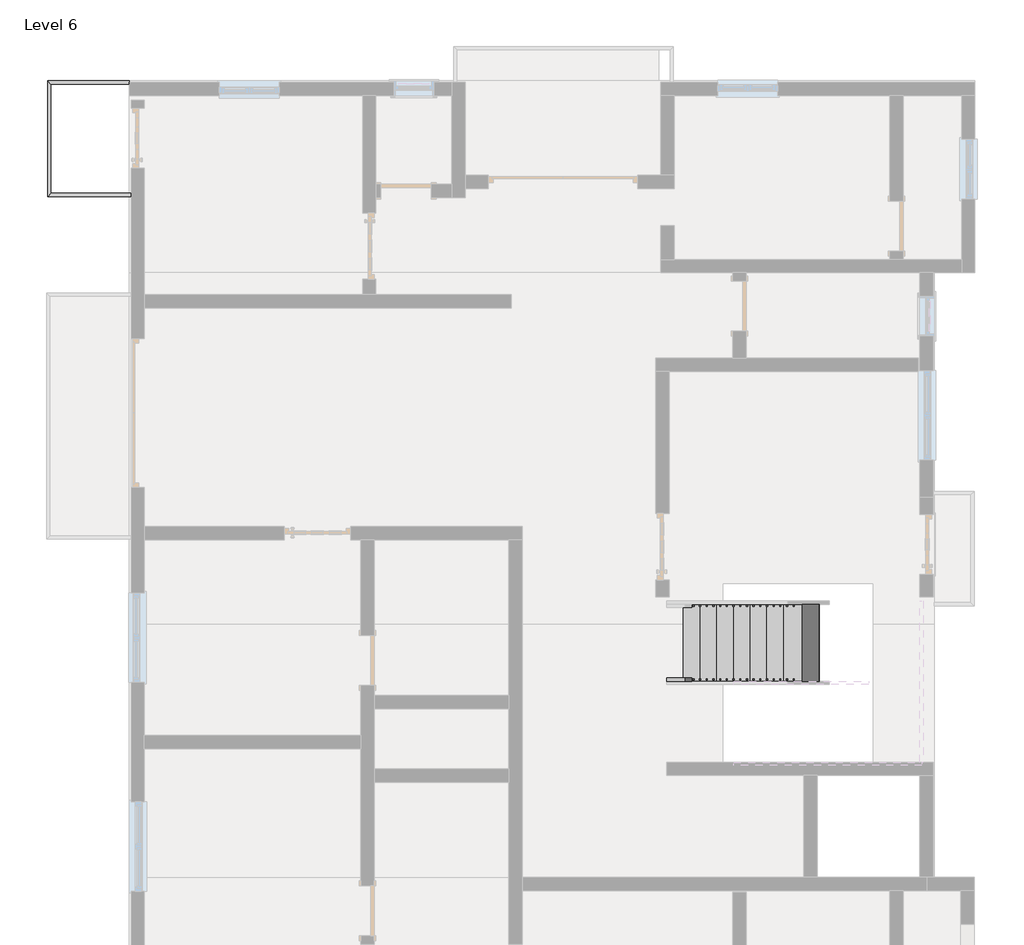
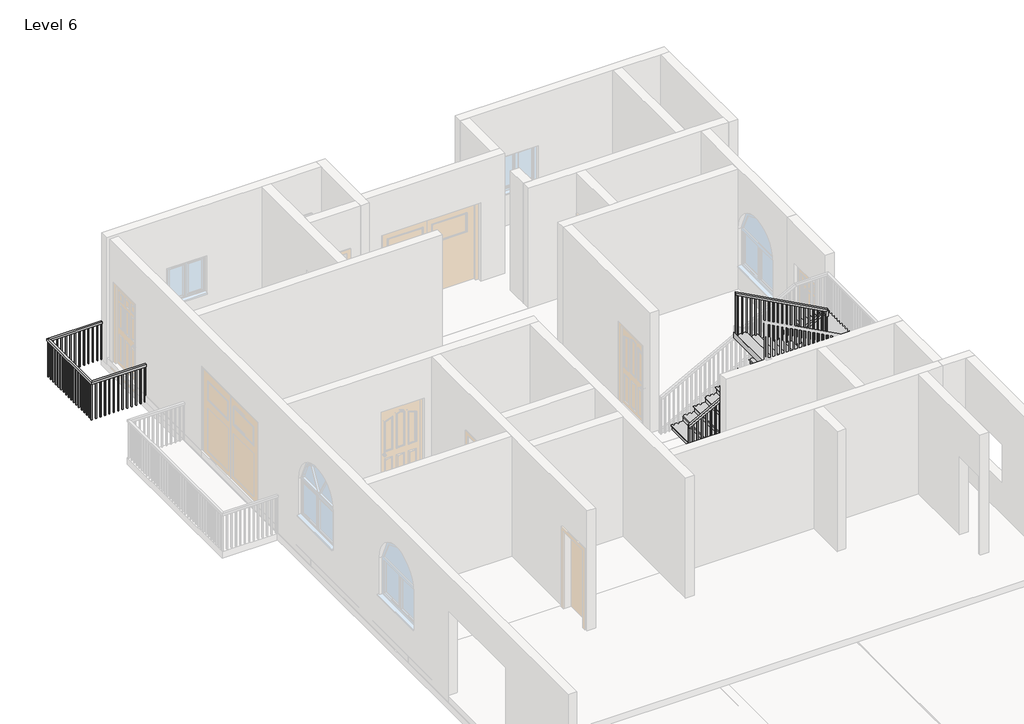
# One storey, part 5 of 7: 2 railings, 1 stair flight.
"""IFC4 building model written with IfcOpenShell, lengths in millimetres."""

from ifc_helpers import new_model, si_unit, frame, origin, place, context, project, spatial, polyline, outline, extrude, faceted_brep, transform, mapped, element, save
from components import stair_flight_0bd31da3

model = new_model("IFC4")

# Units and contexts
model_context = context("Model", 3, world=origin())
ifc_project = project(units=[si_unit("LENGTHUNIT", "METRE", prefix="MILLI")], contexts=[model_context])

# Site, building, storey
site = spatial("IfcSite", under=ifc_project)
building = spatial("IfcBuilding", under=site)
storey = spatial("IfcBuildingStorey", under=building, Name="Level 6", Elevation=15240.0)

# Railings
placement = place(None, origin())
element("IfcRailing", 1, ObjectType="Handrail - Rectangular", at=placement, inside=storey, context=model_context, shape_type="SolidModel", body=[
    faceted_brep([(-6354.2109037, 9376.4527313, 16154.4), (-6354.2109037, 9376.4527313, 16103.6), (-6354.2109037, 9427.2527313, 16103.6), (-6354.2109037, 9427.2527313, 16154.4), (-7548.0109037, 9376.4527313, 16154.4), (-7548.0109037, 9376.4527313, 16103.6), (-7598.8109037, 9427.2527313, 16103.6), (-7598.8109037, 9427.2527313, 16154.4), (-7548.0109037, 7717.9584215, 16154.4), (-7548.0109037, 7717.9584215, 16103.6), (-7598.8109037, 7667.1584215, 16103.6), (-7598.8109037, 7667.1584215, 16154.4), (-6330.8013636, 7717.9584215, 16154.4), (-6330.8013636, 7667.1584215, 16154.4), (-6330.8013636, 7667.1584215, 16103.6), (-6330.8013636, 7717.9584215, 16103.6)], [[[0, 1, 2, 3]], [[1, 0, 4, 5]], [[2, 1, 5, 6]], [[3, 2, 6, 7]], [[0, 3, 7, 4]], [[5, 4, 8, 9]], [[6, 5, 9, 10]], [[7, 6, 10, 11]], [[4, 7, 11, 8]], [[12, 13, 14, 15]], [[9, 8, 12, 15]], [[10, 9, 15, 14]], [[11, 10, 14, 13]], [[8, 11, 13, 12]]]),
    extrude(outline(polyline([(-6363.7359037, 7683.0334215), (-6363.7359037, 7702.0834215), (-6344.6859037, 7702.0834215), (-6344.6859037, 7683.0334215), (-6363.7359037, 7683.0334215)])), frame((0.0, 0.0, 15240.0), z_axis=(0.0, 0.0, 1.0), x_axis=(1.0, 0.0, 0.0)), (0.0, 0.0, 1.0), 863.6),
    extrude(outline(polyline([(-6465.3359037, 7683.0334215), (-6465.3359037, 7702.0834215), (-6446.2859037, 7702.0834215), (-6446.2859037, 7683.0334215), (-6465.3359037, 7683.0334215)])), frame((0.0, 0.0, 15240.0), z_axis=(0.0, 0.0, 1.0), x_axis=(1.0, 0.0, 0.0)), (0.0, 0.0, 1.0), 863.6),
    extrude(outline(polyline([(-6566.9359037, 7683.0334215), (-6566.9359037, 7702.0834215), (-6547.8859037, 7702.0834215), (-6547.8859037, 7683.0334215), (-6566.9359037, 7683.0334215)])), frame((0.0, 0.0, 15240.0), z_axis=(0.0, 0.0, 1.0), x_axis=(1.0, 0.0, 0.0)), (0.0, 0.0, 1.0), 863.6),
    extrude(outline(polyline([(-6668.5359037, 7683.0334215), (-6668.5359037, 7702.0834215), (-6649.4859037, 7702.0834215), (-6649.4859037, 7683.0334215), (-6668.5359037, 7683.0334215)])), frame((0.0, 0.0, 15240.0), z_axis=(0.0, 0.0, 1.0), x_axis=(1.0, 0.0, 0.0)), (0.0, 0.0, 1.0), 863.6),
    extrude(outline(polyline([(-6770.1359037, 7683.0334215), (-6770.1359037, 7702.0834215), (-6751.0859037, 7702.0834215), (-6751.0859037, 7683.0334215), (-6770.1359037, 7683.0334215)])), frame((0.0, 0.0, 15240.0), z_axis=(0.0, 0.0, 1.0), x_axis=(1.0, 0.0, 0.0)), (0.0, 0.0, 1.0), 863.6),
    extrude(outline(polyline([(-6871.7359037, 7683.0334215), (-6871.7359037, 7702.0834215), (-6852.6859037, 7702.0834215), (-6852.6859037, 7683.0334215), (-6871.7359037, 7683.0334215)])), frame((0.0, 0.0, 15240.0), z_axis=(0.0, 0.0, 1.0), x_axis=(1.0, 0.0, 0.0)), (0.0, 0.0, 1.0), 863.6),
    extrude(outline(polyline([(-6973.3359037, 7683.0334215), (-6973.3359037, 7702.0834215), (-6954.2859037, 7702.0834215), (-6954.2859037, 7683.0334215), (-6973.3359037, 7683.0334215)])), frame((0.0, 0.0, 15240.0), z_axis=(0.0, 0.0, 1.0), x_axis=(1.0, 0.0, 0.0)), (0.0, 0.0, 1.0), 863.6),
    extrude(outline(polyline([(-7074.9359037, 7683.0334215), (-7074.9359037, 7702.0834215), (-7055.8859037, 7702.0834215), (-7055.8859037, 7683.0334215), (-7074.9359037, 7683.0334215)])), frame((0.0, 0.0, 15240.0), z_axis=(0.0, 0.0, 1.0), x_axis=(1.0, 0.0, 0.0)), (0.0, 0.0, 1.0), 863.6),
    extrude(outline(polyline([(-7176.5359037, 7683.0334215), (-7176.5359037, 7702.0834215), (-7157.4859037, 7702.0834215), (-7157.4859037, 7683.0334215), (-7176.5359037, 7683.0334215)])), frame((0.0, 0.0, 15240.0), z_axis=(0.0, 0.0, 1.0), x_axis=(1.0, 0.0, 0.0)), (0.0, 0.0, 1.0), 863.6),
    extrude(outline(polyline([(-7278.1359037, 7683.0334215), (-7278.1359037, 7702.0834215), (-7259.0859037, 7702.0834215), (-7259.0859037, 7683.0334215), (-7278.1359037, 7683.0334215)])), frame((0.0, 0.0, 15240.0), z_axis=(0.0, 0.0, 1.0), x_axis=(1.0, 0.0, 0.0)), (0.0, 0.0, 1.0), 863.6),
    extrude(outline(polyline([(-7379.7359037, 7683.0334215), (-7379.7359037, 7702.0834215), (-7360.6859037, 7702.0834215), (-7360.6859037, 7683.0334215), (-7379.7359037, 7683.0334215)])), frame((0.0, 0.0, 15240.0), z_axis=(0.0, 0.0, 1.0), x_axis=(1.0, 0.0, 0.0)), (0.0, 0.0, 1.0), 863.6),
    extrude(outline(polyline([(-7481.3359037, 7683.0334215), (-7481.3359037, 7702.0834215), (-7462.2859037, 7702.0834215), (-7462.2859037, 7683.0334215), (-7481.3359037, 7683.0334215)])), frame((0.0, 0.0, 15240.0), z_axis=(0.0, 0.0, 1.0), x_axis=(1.0, 0.0, 0.0)), (0.0, 0.0, 1.0), 863.6),
    extrude(outline(polyline([(-7582.9359037, 7785.7777313), (-7563.8859037, 7785.7777313), (-7563.8859037, 7766.7277313), (-7582.9359037, 7766.7277313), (-7582.9359037, 7785.7777313)])), frame((0.0, 0.0, 15240.0), z_axis=(0.0, 0.0, 1.0), x_axis=(1.0, 0.0, 0.0)), (0.0, 0.0, 1.0), 863.6),
    extrude(outline(polyline([(-7582.9359037, 7887.3777313), (-7563.8859037, 7887.3777313), (-7563.8859037, 7868.3277313), (-7582.9359037, 7868.3277313), (-7582.9359037, 7887.3777313)])), frame((0.0, 0.0, 15240.0), z_axis=(0.0, 0.0, 1.0), x_axis=(1.0, 0.0, 0.0)), (0.0, 0.0, 1.0), 863.6),
    extrude(outline(polyline([(-7582.9359037, 7988.9777313), (-7563.8859037, 7988.9777313), (-7563.8859037, 7969.9277313), (-7582.9359037, 7969.9277313), (-7582.9359037, 7988.9777313)])), frame((0.0, 0.0, 15240.0), z_axis=(0.0, 0.0, 1.0), x_axis=(1.0, 0.0, 0.0)), (0.0, 0.0, 1.0), 863.6),
    extrude(outline(polyline([(-7582.9359037, 8090.5777313), (-7563.8859037, 8090.5777313), (-7563.8859037, 8071.5277313), (-7582.9359037, 8071.5277313), (-7582.9359037, 8090.5777313)])), frame((0.0, 0.0, 15240.0), z_axis=(0.0, 0.0, 1.0), x_axis=(1.0, 0.0, 0.0)), (0.0, 0.0, 1.0), 863.6),
    extrude(outline(polyline([(-7582.9359037, 8192.1777313), (-7563.8859037, 8192.1777313), (-7563.8859037, 8173.1277313), (-7582.9359037, 8173.1277313), (-7582.9359037, 8192.1777313)])), frame((0.0, 0.0, 15240.0), z_axis=(0.0, 0.0, 1.0), x_axis=(1.0, 0.0, 0.0)), (0.0, 0.0, 1.0), 863.6),
    extrude(outline(polyline([(-7582.9359037, 8293.7777313), (-7563.8859037, 8293.7777313), (-7563.8859037, 8274.7277313), (-7582.9359037, 8274.7277313), (-7582.9359037, 8293.7777313)])), frame((0.0, 0.0, 15240.0), z_axis=(0.0, 0.0, 1.0), x_axis=(1.0, 0.0, 0.0)), (0.0, 0.0, 1.0), 863.6),
    extrude(outline(polyline([(-7582.9359037, 8395.3777313), (-7563.8859037, 8395.3777313), (-7563.8859037, 8376.3277313), (-7582.9359037, 8376.3277313), (-7582.9359037, 8395.3777313)])), frame((0.0, 0.0, 15240.0), z_axis=(0.0, 0.0, 1.0), x_axis=(1.0, 0.0, 0.0)), (0.0, 0.0, 1.0), 863.6),
    extrude(outline(polyline([(-7582.9359037, 8496.9777313), (-7563.8859037, 8496.9777313), (-7563.8859037, 8477.9277313), (-7582.9359037, 8477.9277313), (-7582.9359037, 8496.9777313)])), frame((0.0, 0.0, 15240.0), z_axis=(0.0, 0.0, 1.0), x_axis=(1.0, 0.0, 0.0)), (0.0, 0.0, 1.0), 863.6),
    extrude(outline(polyline([(-7582.9359037, 8598.5777313), (-7563.8859037, 8598.5777313), (-7563.8859037, 8579.5277313), (-7582.9359037, 8579.5277313), (-7582.9359037, 8598.5777313)])), frame((0.0, 0.0, 15240.0), z_axis=(0.0, 0.0, 1.0), x_axis=(1.0, 0.0, 0.0)), (0.0, 0.0, 1.0), 863.6),
    extrude(outline(polyline([(-7582.9359037, 8700.1777313), (-7563.8859037, 8700.1777313), (-7563.8859037, 8681.1277313), (-7582.9359037, 8681.1277313), (-7582.9359037, 8700.1777313)])), frame((0.0, 0.0, 15240.0), z_axis=(0.0, 0.0, 1.0), x_axis=(1.0, 0.0, 0.0)), (0.0, 0.0, 1.0), 863.6),
    extrude(outline(polyline([(-7582.9359037, 8801.7777313), (-7563.8859037, 8801.7777313), (-7563.8859037, 8782.7277313), (-7582.9359037, 8782.7277313), (-7582.9359037, 8801.7777313)])), frame((0.0, 0.0, 15240.0), z_axis=(0.0, 0.0, 1.0), x_axis=(1.0, 0.0, 0.0)), (0.0, 0.0, 1.0), 863.6),
    extrude(outline(polyline([(-7582.9359037, 8903.3777313), (-7563.8859037, 8903.3777313), (-7563.8859037, 8884.3277313), (-7582.9359037, 8884.3277313), (-7582.9359037, 8903.3777313)])), frame((0.0, 0.0, 15240.0), z_axis=(0.0, 0.0, 1.0), x_axis=(1.0, 0.0, 0.0)), (0.0, 0.0, 1.0), 863.6),
    extrude(outline(polyline([(-7582.9359037, 9004.9777313), (-7563.8859037, 9004.9777313), (-7563.8859037, 8985.9277313), (-7582.9359037, 8985.9277313), (-7582.9359037, 9004.9777313)])), frame((0.0, 0.0, 15240.0), z_axis=(0.0, 0.0, 1.0), x_axis=(1.0, 0.0, 0.0)), (0.0, 0.0, 1.0), 863.6),
    extrude(outline(polyline([(-7582.9359037, 9106.5777313), (-7563.8859037, 9106.5777313), (-7563.8859037, 9087.5277313), (-7582.9359037, 9087.5277313), (-7582.9359037, 9106.5777313)])), frame((0.0, 0.0, 15240.0), z_axis=(0.0, 0.0, 1.0), x_axis=(1.0, 0.0, 0.0)), (0.0, 0.0, 1.0), 863.6),
    extrude(outline(polyline([(-7582.9359037, 9208.1777313), (-7563.8859037, 9208.1777313), (-7563.8859037, 9189.1277313), (-7582.9359037, 9189.1277313), (-7582.9359037, 9208.1777313)])), frame((0.0, 0.0, 15240.0), z_axis=(0.0, 0.0, 1.0), x_axis=(1.0, 0.0, 0.0)), (0.0, 0.0, 1.0), 863.6),
    extrude(outline(polyline([(-7582.9359037, 9309.7777313), (-7563.8859037, 9309.7777313), (-7563.8859037, 9290.7277313), (-7582.9359037, 9290.7277313), (-7582.9359037, 9309.7777313)])), frame((0.0, 0.0, 15240.0), z_axis=(0.0, 0.0, 1.0), x_axis=(1.0, 0.0, 0.0)), (0.0, 0.0, 1.0), 863.6),
    extrude(outline(polyline([(-7462.2859037, 9411.3777313), (-7462.2859037, 9392.3277313), (-7481.3359037, 9392.3277313), (-7481.3359037, 9411.3777313), (-7462.2859037, 9411.3777313)])), frame((0.0, 0.0, 15240.0), z_axis=(0.0, 0.0, 1.0), x_axis=(1.0, 0.0, 0.0)), (0.0, 0.0, 1.0), 863.6),
    extrude(outline(polyline([(-7360.6859037, 9411.3777313), (-7360.6859037, 9392.3277313), (-7379.7359037, 9392.3277313), (-7379.7359037, 9411.3777313), (-7360.6859037, 9411.3777313)])), frame((0.0, 0.0, 15240.0), z_axis=(0.0, 0.0, 1.0), x_axis=(1.0, 0.0, 0.0)), (0.0, 0.0, 1.0), 863.6),
    extrude(outline(polyline([(-7259.0859037, 9411.3777313), (-7259.0859037, 9392.3277313), (-7278.1359037, 9392.3277313), (-7278.1359037, 9411.3777313), (-7259.0859037, 9411.3777313)])), frame((0.0, 0.0, 15240.0), z_axis=(0.0, 0.0, 1.0), x_axis=(1.0, 0.0, 0.0)), (0.0, 0.0, 1.0), 863.6),
    extrude(outline(polyline([(-7157.4859037, 9411.3777313), (-7157.4859037, 9392.3277313), (-7176.5359037, 9392.3277313), (-7176.5359037, 9411.3777313), (-7157.4859037, 9411.3777313)])), frame((0.0, 0.0, 15240.0), z_axis=(0.0, 0.0, 1.0), x_axis=(1.0, 0.0, 0.0)), (0.0, 0.0, 1.0), 863.6),
    extrude(outline(polyline([(-7055.8859037, 9411.3777313), (-7055.8859037, 9392.3277313), (-7074.9359037, 9392.3277313), (-7074.9359037, 9411.3777313), (-7055.8859037, 9411.3777313)])), frame((0.0, 0.0, 15240.0), z_axis=(0.0, 0.0, 1.0), x_axis=(1.0, 0.0, 0.0)), (0.0, 0.0, 1.0), 863.6),
    extrude(outline(polyline([(-6954.2859037, 9411.3777313), (-6954.2859037, 9392.3277313), (-6973.3359037, 9392.3277313), (-6973.3359037, 9411.3777313), (-6954.2859037, 9411.3777313)])), frame((0.0, 0.0, 15240.0), z_axis=(0.0, 0.0, 1.0), x_axis=(1.0, 0.0, 0.0)), (0.0, 0.0, 1.0), 863.6),
    extrude(outline(polyline([(-6852.6859037, 9411.3777313), (-6852.6859037, 9392.3277313), (-6871.7359037, 9392.3277313), (-6871.7359037, 9411.3777313), (-6852.6859037, 9411.3777313)])), frame((0.0, 0.0, 15240.0), z_axis=(0.0, 0.0, 1.0), x_axis=(1.0, 0.0, 0.0)), (0.0, 0.0, 1.0), 863.6),
    extrude(outline(polyline([(-6751.0859037, 9411.3777313), (-6751.0859037, 9392.3277313), (-6770.1359037, 9392.3277313), (-6770.1359037, 9411.3777313), (-6751.0859037, 9411.3777313)])), frame((0.0, 0.0, 15240.0), z_axis=(0.0, 0.0, 1.0), x_axis=(1.0, 0.0, 0.0)), (0.0, 0.0, 1.0), 863.6),
    extrude(outline(polyline([(-6649.4859037, 9411.3777313), (-6649.4859037, 9392.3277313), (-6668.5359037, 9392.3277313), (-6668.5359037, 9411.3777313), (-6649.4859037, 9411.3777313)])), frame((0.0, 0.0, 15240.0), z_axis=(0.0, 0.0, 1.0), x_axis=(1.0, 0.0, 0.0)), (0.0, 0.0, 1.0), 863.6),
    extrude(outline(polyline([(-6547.8859037, 9411.3777313), (-6547.8859037, 9392.3277313), (-6566.9359037, 9392.3277313), (-6566.9359037, 9411.3777313), (-6547.8859037, 9411.3777313)])), frame((0.0, 0.0, 15240.0), z_axis=(0.0, 0.0, 1.0), x_axis=(1.0, 0.0, 0.0)), (0.0, 0.0, 1.0), 863.6),
    extrude(outline(polyline([(-6446.2859037, 9411.3777313), (-6446.2859037, 9392.3277313), (-6465.3359037, 9392.3277313), (-6465.3359037, 9411.3777313), (-6446.2859037, 9411.3777313)])), frame((0.0, 0.0, 15240.0), z_axis=(0.0, 0.0, 1.0), x_axis=(1.0, 0.0, 0.0)), (0.0, 0.0, 1.0), 863.6),
    extrude(outline(polyline([(-7582.9359037, 7702.0834215), (-7563.8859037, 7702.0834215), (-7563.8859037, 7683.0334215), (-7582.9359037, 7683.0334215), (-7582.9359037, 7702.0834215)])), frame((0.0, 0.0, 15240.0), z_axis=(0.0, 0.0, 1.0), x_axis=(1.0, 0.0, 0.0)), (0.0, 0.0, 1.0), 863.6),
    extrude(outline(polyline([(-7563.8859037, 9411.3777313), (-7563.8859037, 9392.3277313), (-7582.9359037, 9392.3277313), (-7582.9359037, 9411.3777313), (-7563.8859037, 9411.3777313)])), frame((0.0, 0.0, 15240.0), z_axis=(0.0, 0.0, 1.0), x_axis=(1.0, 0.0, 0.0)), (0.0, 0.0, 1.0), 863.6),
    extrude(outline(polyline([(-6349.8513636, 7683.0334215), (-6349.8513636, 7702.0834215), (-6330.8013636, 7702.0834215), (-6330.8013636, 7683.0334215), (-6349.8513636, 7683.0334215)])), frame((0.0, 0.0, 15240.0), z_axis=(0.0, 0.0, 1.0), x_axis=(1.0, 0.0, 0.0)), (0.0, 0.0, 1.0), 863.6),
    extrude(outline(polyline([(-6354.2109037, 9411.3777313), (-6354.2109037, 9392.3277313), (-6373.2609037, 9392.3277313), (-6373.2609037, 9411.3777313), (-6354.2109037, 9411.3777313)])), frame((0.0, 0.0, 15240.0), z_axis=(0.0, 0.0, 1.0), x_axis=(1.0, 0.0, 0.0)), (0.0, 0.0, 1.0), 863.6),
])
element("IfcRailing", 2, ObjectType="Handrail - Rectangular", at=placement, inside=storey, context=model_context, shape_type="SolidModel", body=[
    faceted_brep([(1811.8890963, 347.1962251, 16292.9454545), (1811.8890963, 347.1962251, 16235.1709673), (1811.8890963, 296.3962251, 16235.1709673), (1811.8890963, 296.3962251, 16292.9454545), (4804.8326586, 347.1962251, 17914.2136078), (4855.6326586, 347.1962251, 17883.9573214), (4855.6326586, 296.3962251, 17883.9573214), (4804.8326586, 296.3962251, 17914.2136078), (4804.8326586, 347.1962251, 17955.4909091), (4855.6326586, 347.1962251, 17904.6909091), (4855.6326586, 296.3962251, 17904.6909091), (4804.8326586, 296.3962251, 17955.4909091), (4931.8326586, 347.1962251, 17955.4909091), (4931.8326586, 347.1962251, 17904.6909091), (4881.0326586, 296.3962251, 17904.6909091), (4881.0326586, 296.3962251, 17955.4909091), (4931.8326586, 245.5962251, 17955.4909091), (4881.0326586, 245.5962251, 17955.4909091), (4881.0326586, 194.7962251, 17904.6909091), (4931.8326586, 194.7962251, 17904.6909091)], [[[0, 1, 2, 3]], [[1, 0, 4, 5]], [[2, 1, 5, 6]], [[3, 2, 6, 7]], [[0, 3, 7, 4]], [[5, 4, 8, 9]], [[6, 5, 9, 10]], [[7, 6, 10, 11]], [[4, 7, 11, 8]], [[9, 8, 12, 13]], [[10, 9, 13, 14]], [[11, 10, 14, 15]], [[8, 11, 15, 12]], [[16, 17, 18, 19]], [[13, 12, 16, 19]], [[14, 13, 19, 18]], [[15, 14, 18, 17]], [[12, 15, 17, 16]]]),
    faceted_brep([(4931.8326586, 245.5962251, 17955.4909091), (4931.8326586, 194.7962251, 17904.6909091), (4881.0326586, 194.7962251, 17904.6909091), (4881.0326586, 245.5962251, 17955.4909091), (4931.8326586, 245.5962251, 18066.6126249), (4881.0326586, 245.5962251, 18036.3068093), (4881.0326586, 194.7962251, 18036.3068093), (4931.8326586, 194.7962251, 18066.6126249)], [[[0, 1, 2, 3]], [[4, 5, 6, 7]], [[1, 0, 4, 7]], [[2, 1, 7, 6]], [[3, 2, 6, 5]], [[0, 3, 5, 4]]]),
    faceted_brep([(4931.8326586, 194.7962251, 18066.6126249), (4881.0326586, 194.7962251, 18036.3068093), (4881.0326586, 245.5962251, 18036.3068093), (4931.8326586, 245.5962251, 18066.6126249), (2827.8890963, 194.7962251, 19202.4), (2827.8890963, 245.5962251, 19202.4), (2827.8890963, 245.5962251, 19144.6704456), (2827.8890963, 194.7962251, 19144.6704456)], [[[0, 1, 2, 3]], [[4, 5, 6, 7]], [[1, 0, 4, 7]], [[2, 1, 7, 6]], [[3, 2, 6, 5]], [[0, 3, 5, 4]]]),
    extrude(outline(polyline([(19114.40254, 2883.9576586), (19124.686442, 2864.9076586), (18149.4545455, 2864.9076586), (18149.4545455, 2883.9576586), (19114.40254, 2883.9576586)])), frame((0.0, 210.6712251, 0.0), z_axis=(0.0, 1.0, 0.0), x_axis=(0.0, 0.0, 1.0)), (0.0, 0.0, 1.0), 19.05),
    extrude(outline(polyline([(19059.5550624, 2985.5576586), (19069.8389645, 2966.5076586), (18149.4545455, 2966.5076586), (18149.4545455, 2985.5576586), (19059.5550624, 2985.5576586)])), frame((0.0, 210.6712251, 0.0), z_axis=(0.0, 1.0, 0.0), x_axis=(0.0, 0.0, 1.0)), (0.0, 0.0, 1.0), 19.05),
    extrude(outline(polyline([(19004.7075849, 3087.1576586), (19014.9914869, 3068.1076586), (18149.4545455, 3068.1076586), (18149.4545455, 3087.1576586), (19004.7075849, 3087.1576586)])), frame((0.0, 210.6712251, 0.0), z_axis=(0.0, 1.0, 0.0), x_axis=(0.0, 0.0, 1.0)), (0.0, 0.0, 1.0), 19.05),
    extrude(outline(polyline([(18949.8601073, 3188.7576586), (18960.1440094, 3169.7076586), (18010.9090909, 3169.7076586), (18010.9090909, 3188.7576586), (18949.8601073, 3188.7576586)])), frame((0.0, 210.6712251, 0.0), z_axis=(0.0, 1.0, 0.0), x_axis=(0.0, 0.0, 1.0)), (0.0, 0.0, 1.0), 19.05),
    extrude(outline(polyline([(18895.0126298, 3290.3576586), (18905.2965318, 3271.3076586), (18010.9090909, 3271.3076586), (18010.9090909, 3290.3576586), (18895.0126298, 3290.3576586)])), frame((0.0, 210.6712251, 0.0), z_axis=(0.0, 1.0, 0.0), x_axis=(0.0, 0.0, 1.0)), (0.0, 0.0, 1.0), 19.05),
    extrude(outline(polyline([(18840.1651522, 3391.9576586), (18850.4490542, 3372.9076586), (17872.3636364, 3372.9076586), (17872.3636364, 3391.9576586), (18840.1651522, 3391.9576586)])), frame((0.0, 210.6712251, 0.0), z_axis=(0.0, 1.0, 0.0), x_axis=(0.0, 0.0, 1.0)), (0.0, 0.0, 1.0), 19.05),
    extrude(outline(polyline([(18785.3176746, 3493.5576586), (18795.6015767, 3474.5076586), (17872.3636364, 3474.5076586), (17872.3636364, 3493.5576586), (18785.3176746, 3493.5576586)])), frame((0.0, 210.6712251, 0.0), z_axis=(0.0, 1.0, 0.0), x_axis=(0.0, 0.0, 1.0)), (0.0, 0.0, 1.0), 19.05),
    extrude(outline(polyline([(18730.4701971, 3595.1576586), (18740.7540991, 3576.1076586), (17872.3636364, 3576.1076586), (17872.3636364, 3595.1576586), (18730.4701971, 3595.1576586)])), frame((0.0, 210.6712251, 0.0), z_axis=(0.0, 1.0, 0.0), x_axis=(0.0, 0.0, 1.0)), (0.0, 0.0, 1.0), 19.05),
    extrude(outline(polyline([(18675.6227195, 3696.7576586), (18685.9066216, 3677.7076586), (17733.8181818, 3677.7076586), (17733.8181818, 3696.7576586), (18675.6227195, 3696.7576586)])), frame((0.0, 210.6712251, 0.0), z_axis=(0.0, 1.0, 0.0), x_axis=(0.0, 0.0, 1.0)), (0.0, 0.0, 1.0), 19.05),
    extrude(outline(polyline([(18620.775242, 3798.3576586), (18631.059144, 3779.3076586), (17733.8181818, 3779.3076586), (17733.8181818, 3798.3576586), (18620.775242, 3798.3576586)])), frame((0.0, 210.6712251, 0.0), z_axis=(0.0, 1.0, 0.0), x_axis=(0.0, 0.0, 1.0)), (0.0, 0.0, 1.0), 19.05),
    extrude(outline(polyline([(18565.9277644, 3899.9576586), (18576.2116665, 3880.9076586), (17595.2727273, 3880.9076586), (17595.2727273, 3899.9576586), (18565.9277644, 3899.9576586)])), frame((0.0, 210.6712251, 0.0), z_axis=(0.0, 1.0, 0.0), x_axis=(0.0, 0.0, 1.0)), (0.0, 0.0, 1.0), 19.05),
    extrude(outline(polyline([(18511.0802869, 4001.5576586), (18521.3641889, 3982.5076586), (17595.2727273, 3982.5076586), (17595.2727273, 4001.5576586), (18511.0802869, 4001.5576586)])), frame((0.0, 210.6712251, 0.0), z_axis=(0.0, 1.0, 0.0), x_axis=(0.0, 0.0, 1.0)), (0.0, 0.0, 1.0), 19.05),
    extrude(outline(polyline([(18456.2328093, 4103.1576586), (18466.5167113, 4084.1076586), (17595.2727273, 4084.1076586), (17595.2727273, 4103.1576586), (18456.2328093, 4103.1576586)])), frame((0.0, 210.6712251, 0.0), z_axis=(0.0, 1.0, 0.0), x_axis=(0.0, 0.0, 1.0)), (0.0, 0.0, 1.0), 19.05),
    extrude(outline(polyline([(18401.3853317, 4204.7576586), (18411.6692338, 4185.7076586), (17456.7272727, 4185.7076586), (17456.7272727, 4204.7576586), (18401.3853317, 4204.7576586)])), frame((0.0, 210.6712251, 0.0), z_axis=(0.0, 1.0, 0.0), x_axis=(0.0, 0.0, 1.0)), (0.0, 0.0, 1.0), 19.05),
    extrude(outline(polyline([(18346.5378542, 4306.3576586), (18356.8217562, 4287.3076586), (17456.7272727, 4287.3076586), (17456.7272727, 4306.3576586), (18346.5378542, 4306.3576586)])), frame((0.0, 210.6712251, 0.0), z_axis=(0.0, 1.0, 0.0), x_axis=(0.0, 0.0, 1.0)), (0.0, 0.0, 1.0), 19.05),
    extrude(outline(polyline([(18291.6903766, 4407.9576586), (18301.9742787, 4388.9076586), (17318.1818182, 4388.9076586), (17318.1818182, 4407.9576586), (18291.6903766, 4407.9576586)])), frame((0.0, 210.6712251, 0.0), z_axis=(0.0, 1.0, 0.0), x_axis=(0.0, 0.0, 1.0)), (0.0, 0.0, 1.0), 19.05),
    extrude(outline(polyline([(18236.8428991, 4509.5576586), (18247.1268011, 4490.5076586), (17318.1818182, 4490.5076586), (17318.1818182, 4509.5576586), (18236.8428991, 4509.5576586)])), frame((0.0, 210.6712251, 0.0), z_axis=(0.0, 1.0, 0.0), x_axis=(0.0, 0.0, 1.0)), (0.0, 0.0, 1.0), 19.05),
    extrude(outline(polyline([(18181.9954215, 4611.1576586), (18192.2793236, 4592.1076586), (17318.1818182, 4592.1076586), (17318.1818182, 4611.1576586), (18181.9954215, 4611.1576586)])), frame((0.0, 210.6712251, 0.0), z_axis=(0.0, 1.0, 0.0), x_axis=(0.0, 0.0, 1.0)), (0.0, 0.0, 1.0), 19.05),
    extrude(outline(polyline([(18127.147944, 4712.7576586), (18137.431846, 4693.7076586), (17179.6363636, 4693.7076586), (17179.6363636, 4712.7576586), (18127.147944, 4712.7576586)])), frame((0.0, 210.6712251, 0.0), z_axis=(0.0, 1.0, 0.0), x_axis=(0.0, 0.0, 1.0)), (0.0, 0.0, 1.0), 19.05),
    extrude(outline(polyline([(18072.3004664, 4814.3576586), (18082.5843684, 4795.3076586), (17179.6363636, 4795.3076586), (17179.6363636, 4814.3576586), (18072.3004664, 4814.3576586)])), frame((0.0, 210.6712251, 0.0), z_axis=(0.0, 1.0, 0.0), x_axis=(0.0, 0.0, 1.0)), (0.0, 0.0, 1.0), 19.05),
    extrude(outline(polyline([(4850.3640963, 312.2712251), (4850.3640963, 331.3212251), (4869.4140963, 331.3212251), (4869.4140963, 312.2712251), (4850.3640963, 312.2712251)])), frame((0.0, 0.0, 16902.5454545), z_axis=(0.0, 0.0, 1.0), x_axis=(1.0, 0.0, 0.0)), (0.0, 0.0, 1.0), 1002.1454545),
    extrude(outline(polyline([(17836.3862812, 4767.8140963), (17826.0669559, 4748.7640963), (16902.5454545, 4748.7640963), (16902.5454545, 4767.8140963), (17836.3862812, 4767.8140963)])), frame((0.0, 312.2712251, 0.0), z_axis=(0.0, 1.0, 0.0), x_axis=(0.0, 0.0, 1.0)), (0.0, 0.0, 1.0), 19.05),
    extrude(outline(polyline([(17781.3498795, 4666.2140963), (17771.0305541, 4647.1640963), (16902.5454545, 4647.1640963), (16902.5454545, 4666.2140963), (17781.3498795, 4666.2140963)])), frame((0.0, 312.2712251, 0.0), z_axis=(0.0, 1.0, 0.0), x_axis=(0.0, 0.0, 1.0)), (0.0, 0.0, 1.0), 19.05),
    extrude(outline(polyline([(17726.3134777, 4564.6140963), (17715.9941524, 4545.5640963), (16764.0, 4545.5640963), (16764.0, 4564.6140963), (17726.3134777, 4564.6140963)])), frame((0.0, 312.2712251, 0.0), z_axis=(0.0, 1.0, 0.0), x_axis=(0.0, 0.0, 1.0)), (0.0, 0.0, 1.0), 19.05),
    extrude(outline(polyline([(17671.2770759, 4463.0140963), (17660.9577506, 4443.9640963), (16764.0, 4443.9640963), (16764.0, 4463.0140963), (17671.2770759, 4463.0140963)])), frame((0.0, 312.2712251, 0.0), z_axis=(0.0, 1.0, 0.0), x_axis=(0.0, 0.0, 1.0)), (0.0, 0.0, 1.0), 19.05),
    extrude(outline(polyline([(17616.2406742, 4361.4140963), (17605.9213488, 4342.3640963), (16764.0, 4342.3640963), (16764.0, 4361.4140963), (17616.2406742, 4361.4140963)])), frame((0.0, 312.2712251, 0.0), z_axis=(0.0, 1.0, 0.0), x_axis=(0.0, 0.0, 1.0)), (0.0, 0.0, 1.0), 19.05),
    extrude(outline(polyline([(17561.2042724, 4259.8140963), (17550.8849471, 4240.7640963), (16625.4545455, 4240.7640963), (16625.4545455, 4259.8140963), (17561.2042724, 4259.8140963)])), frame((0.0, 312.2712251, 0.0), z_axis=(0.0, 1.0, 0.0), x_axis=(0.0, 0.0, 1.0)), (0.0, 0.0, 1.0), 19.05),
    extrude(outline(polyline([(17506.1678706, 4158.2140963), (17495.8485453, 4139.1640963), (16625.4545455, 4139.1640963), (16625.4545455, 4158.2140963), (17506.1678706, 4158.2140963)])), frame((0.0, 312.2712251, 0.0), z_axis=(0.0, 1.0, 0.0), x_axis=(0.0, 0.0, 1.0)), (0.0, 0.0, 1.0), 19.05),
    extrude(outline(polyline([(17451.1314688, 4056.6140963), (17440.8121435, 4037.5640963), (16486.9090909, 4037.5640963), (16486.9090909, 4056.6140963), (17451.1314688, 4056.6140963)])), frame((0.0, 312.2712251, 0.0), z_axis=(0.0, 1.0, 0.0), x_axis=(0.0, 0.0, 1.0)), (0.0, 0.0, 1.0), 19.05),
    extrude(outline(polyline([(17396.0950671, 3955.0140963), (17385.7757417, 3935.9640963), (16486.9090909, 3935.9640963), (16486.9090909, 3955.0140963), (17396.0950671, 3955.0140963)])), frame((0.0, 312.2712251, 0.0), z_axis=(0.0, 1.0, 0.0), x_axis=(0.0, 0.0, 1.0)), (0.0, 0.0, 1.0), 19.05),
    extrude(outline(polyline([(17341.0586653, 3853.4140963), (17330.73934, 3834.3640963), (16486.9090909, 3834.3640963), (16486.9090909, 3853.4140963), (17341.0586653, 3853.4140963)])), frame((0.0, 312.2712251, 0.0), z_axis=(0.0, 1.0, 0.0), x_axis=(0.0, 0.0, 1.0)), (0.0, 0.0, 1.0), 19.05),
    extrude(outline(polyline([(17286.0222635, 3751.8140963), (17275.7029382, 3732.7640963), (16348.3636364, 3732.7640963), (16348.3636364, 3751.8140963), (17286.0222635, 3751.8140963)])), frame((0.0, 312.2712251, 0.0), z_axis=(0.0, 1.0, 0.0), x_axis=(0.0, 0.0, 1.0)), (0.0, 0.0, 1.0), 19.05),
    extrude(outline(polyline([(17230.9858618, 3650.2140963), (17220.6665364, 3631.1640963), (16348.3636364, 3631.1640963), (16348.3636364, 3650.2140963), (17230.9858618, 3650.2140963)])), frame((0.0, 312.2712251, 0.0), z_axis=(0.0, 1.0, 0.0), x_axis=(0.0, 0.0, 1.0)), (0.0, 0.0, 1.0), 19.05),
    extrude(outline(polyline([(17175.94946, 3548.6140963), (17165.6301347, 3529.5640963), (16209.8181818, 3529.5640963), (16209.8181818, 3548.6140963), (17175.94946, 3548.6140963)])), frame((0.0, 312.2712251, 0.0), z_axis=(0.0, 1.0, 0.0), x_axis=(0.0, 0.0, 1.0)), (0.0, 0.0, 1.0), 19.05),
    extrude(outline(polyline([(17120.9130582, 3447.0140963), (17110.5937329, 3427.9640963), (16209.8181818, 3427.9640963), (16209.8181818, 3447.0140963), (17120.9130582, 3447.0140963)])), frame((0.0, 312.2712251, 0.0), z_axis=(0.0, 1.0, 0.0), x_axis=(0.0, 0.0, 1.0)), (0.0, 0.0, 1.0), 19.05),
    extrude(outline(polyline([(17065.8766565, 3345.4140963), (17055.5573311, 3326.3640963), (16209.8181818, 3326.3640963), (16209.8181818, 3345.4140963), (17065.8766565, 3345.4140963)])), frame((0.0, 312.2712251, 0.0), z_axis=(0.0, 1.0, 0.0), x_axis=(0.0, 0.0, 1.0)), (0.0, 0.0, 1.0), 19.05),
    extrude(outline(polyline([(17010.8402547, 3243.8140963), (17000.5209294, 3224.7640963), (16071.2727273, 3224.7640963), (16071.2727273, 3243.8140963), (17010.8402547, 3243.8140963)])), frame((0.0, 312.2712251, 0.0), z_axis=(0.0, 1.0, 0.0), x_axis=(0.0, 0.0, 1.0)), (0.0, 0.0, 1.0), 19.05),
    extrude(outline(polyline([(16955.8038529, 3142.2140963), (16945.4845276, 3123.1640963), (16071.2727273, 3123.1640963), (16071.2727273, 3142.2140963), (16955.8038529, 3142.2140963)])), frame((0.0, 312.2712251, 0.0), z_axis=(0.0, 1.0, 0.0), x_axis=(0.0, 0.0, 1.0)), (0.0, 0.0, 1.0), 19.05),
    extrude(outline(polyline([(16900.7674512, 3040.6140963), (16890.4481258, 3021.5640963), (15932.7272727, 3021.5640963), (15932.7272727, 3040.6140963), (16900.7674512, 3040.6140963)])), frame((0.0, 312.2712251, 0.0), z_axis=(0.0, 1.0, 0.0), x_axis=(0.0, 0.0, 1.0)), (0.0, 0.0, 1.0), 19.05),
    extrude(outline(polyline([(16845.7310494, 2939.0140963), (16835.4117241, 2919.9640963), (15932.7272727, 2919.9640963), (15932.7272727, 2939.0140963), (16845.7310494, 2939.0140963)])), frame((0.0, 312.2712251, 0.0), z_axis=(0.0, 1.0, 0.0), x_axis=(0.0, 0.0, 1.0)), (0.0, 0.0, 1.0), 19.05),
    extrude(outline(polyline([(16790.6946476, 2837.4140963), (16780.3753223, 2818.3640963), (15932.7272727, 2818.3640963), (15932.7272727, 2837.4140963), (16790.6946476, 2837.4140963)])), frame((0.0, 312.2712251, 0.0), z_axis=(0.0, 1.0, 0.0), x_axis=(0.0, 0.0, 1.0)), (0.0, 0.0, 1.0), 19.05),
    extrude(outline(polyline([(16735.6582459, 2735.8140963), (16725.3389205, 2716.7640963), (15794.1818182, 2716.7640963), (15794.1818182, 2735.8140963), (16735.6582459, 2735.8140963)])), frame((0.0, 312.2712251, 0.0), z_axis=(0.0, 1.0, 0.0), x_axis=(0.0, 0.0, 1.0)), (0.0, 0.0, 1.0), 19.05),
    extrude(outline(polyline([(16680.6218441, 2634.2140963), (16670.3025188, 2615.1640963), (15794.1818182, 2615.1640963), (15794.1818182, 2634.2140963), (16680.6218441, 2634.2140963)])), frame((0.0, 312.2712251, 0.0), z_axis=(0.0, 1.0, 0.0), x_axis=(0.0, 0.0, 1.0)), (0.0, 0.0, 1.0), 19.05),
    extrude(outline(polyline([(16625.5854423, 2532.6140963), (16615.266117, 2513.5640963), (15655.6363636, 2513.5640963), (15655.6363636, 2532.6140963), (16625.5854423, 2532.6140963)])), frame((0.0, 312.2712251, 0.0), z_axis=(0.0, 1.0, 0.0), x_axis=(0.0, 0.0, 1.0)), (0.0, 0.0, 1.0), 19.05),
    extrude(outline(polyline([(16570.5490405, 2431.0140963), (16560.2297152, 2411.9640963), (15655.6363636, 2411.9640963), (15655.6363636, 2431.0140963), (16570.5490405, 2431.0140963)])), frame((0.0, 312.2712251, 0.0), z_axis=(0.0, 1.0, 0.0), x_axis=(0.0, 0.0, 1.0)), (0.0, 0.0, 1.0), 19.05),
    extrude(outline(polyline([(16515.5126388, 2329.4140963), (16505.1933134, 2310.3640963), (15655.6363636, 2310.3640963), (15655.6363636, 2329.4140963), (16515.5126388, 2329.4140963)])), frame((0.0, 312.2712251, 0.0), z_axis=(0.0, 1.0, 0.0), x_axis=(0.0, 0.0, 1.0)), (0.0, 0.0, 1.0), 19.05),
    extrude(outline(polyline([(16460.476237, 2227.8140963), (16450.1569117, 2208.7640963), (15517.0909091, 2208.7640963), (15517.0909091, 2227.8140963), (16460.476237, 2227.8140963)])), frame((0.0, 312.2712251, 0.0), z_axis=(0.0, 1.0, 0.0), x_axis=(0.0, 0.0, 1.0)), (0.0, 0.0, 1.0), 19.05),
    extrude(outline(polyline([(16405.4398352, 2126.2140963), (16395.1205099, 2107.1640963), (15517.0909091, 2107.1640963), (15517.0909091, 2126.2140963), (16405.4398352, 2126.2140963)])), frame((0.0, 312.2712251, 0.0), z_axis=(0.0, 1.0, 0.0), x_axis=(0.0, 0.0, 1.0)), (0.0, 0.0, 1.0), 19.05),
    extrude(outline(polyline([(16350.4034335, 2024.6140963), (16340.0841081, 2005.5640963), (15378.5454545, 2005.5640963), (15378.5454545, 2024.6140963), (16350.4034335, 2024.6140963)])), frame((0.0, 312.2712251, 0.0), z_axis=(0.0, 1.0, 0.0), x_axis=(0.0, 0.0, 1.0)), (0.0, 0.0, 1.0), 19.05),
    extrude(outline(polyline([(16295.3670317, 1923.0140963), (16285.0477064, 1903.9640963), (15378.5454545, 1903.9640963), (15378.5454545, 1923.0140963), (16295.3670317, 1923.0140963)])), frame((0.0, 312.2712251, 0.0), z_axis=(0.0, 1.0, 0.0), x_axis=(0.0, 0.0, 1.0)), (0.0, 0.0, 1.0), 19.05),
    extrude(outline(polyline([(4896.9076586, 229.7212251), (4915.9576586, 229.7212251), (4915.9576586, 210.6712251), (4896.9076586, 210.6712251), (4896.9076586, 229.7212251)])), frame((0.0, 0.0, 17041.0909091), z_axis=(0.0, 0.0, 1.0), x_axis=(1.0, 0.0, 0.0)), (0.0, 0.0, 1.0), 863.6),
    extrude(outline(polyline([(4896.9076586, 312.2712251), (4896.9076586, 331.3212251), (4915.9576586, 331.3212251), (4915.9576586, 312.2712251), (4896.9076586, 312.2712251)])), frame((0.0, 0.0, 17041.0909091), z_axis=(0.0, 0.0, 1.0), x_axis=(1.0, 0.0, 0.0)), (0.0, 0.0, 1.0), 863.6),
    extrude(outline(polyline([(19134.3865436, 2846.9390963), (19144.6704456, 2827.8890963), (18149.4545455, 2827.8890963), (18149.4545455, 2846.9390963), (19134.3865436, 2846.9390963)])), frame((0.0, 210.6712251, 0.0), z_axis=(0.0, 1.0, 0.0), x_axis=(0.0, 0.0, 1.0)), (0.0, 0.0, 1.0), 19.05),
    extrude(outline(polyline([(16245.4902926, 1830.9390963), (16235.1709673, 1811.8890963), (15378.5454545, 1811.8890963), (15378.5454545, 1830.9390963), (16245.4902926, 1830.9390963)])), frame((0.0, 312.2712251, 0.0), z_axis=(0.0, 1.0, 0.0), x_axis=(0.0, 0.0, 1.0)), (0.0, 0.0, 1.0), 19.05),
])

# Stair flight
stair_flight_shape = stair_flight_0bd31da3(model_context)
element("IfcStairFlight", 3, ObjectType="2\" Tread 1\" Nosing 1/4\" Riser", at=placement, inside=storey, context=model_context, shape_type="MappedRepresentation", body=[
    mapped(stair_flight_shape, transform((0.0, 0.0, 0.0), x_axis=(1.0, 0.0, 0.0), y_axis=(0.0, 1.0, 0.0), z_axis=(0.0, 0.0, 1.0))),
])

save(model, "model.ifc")

# Revit data of these elements
# Type "Handrail - Rectangular"
#   Assembly Code = "C2010400"
#   built-in parameter 1008612 = 0.0416667 (stored number, unit not read)
#   built-in parameter 1008611 = 0.0416667 (stored number, unit not read)
#   built-in parameter 1008609 = 0.333333 (stored number, unit not read)
#   built-in parameter 1008604 = 0.166667 (stored number, unit not read)
#   built-in parameter 1008603 = 0.166667 (stored number, unit not read)
#   Railing Height = 3' - 0"
#   built-in parameter 1008630 = 2
#   built-in parameter 1008610 = 2
#   built-in parameter 1008618 = Baluster - Square : 3/4"
# Elements 1, 2 (IfcRailing, "Handrail - Rectangular")
#   Phase Created = New Construction
# Element 3 (IfcStairFlight, "2\" Tread 1\" Nosing 1/4\" Riser")
#   Phase Created = New Construction
